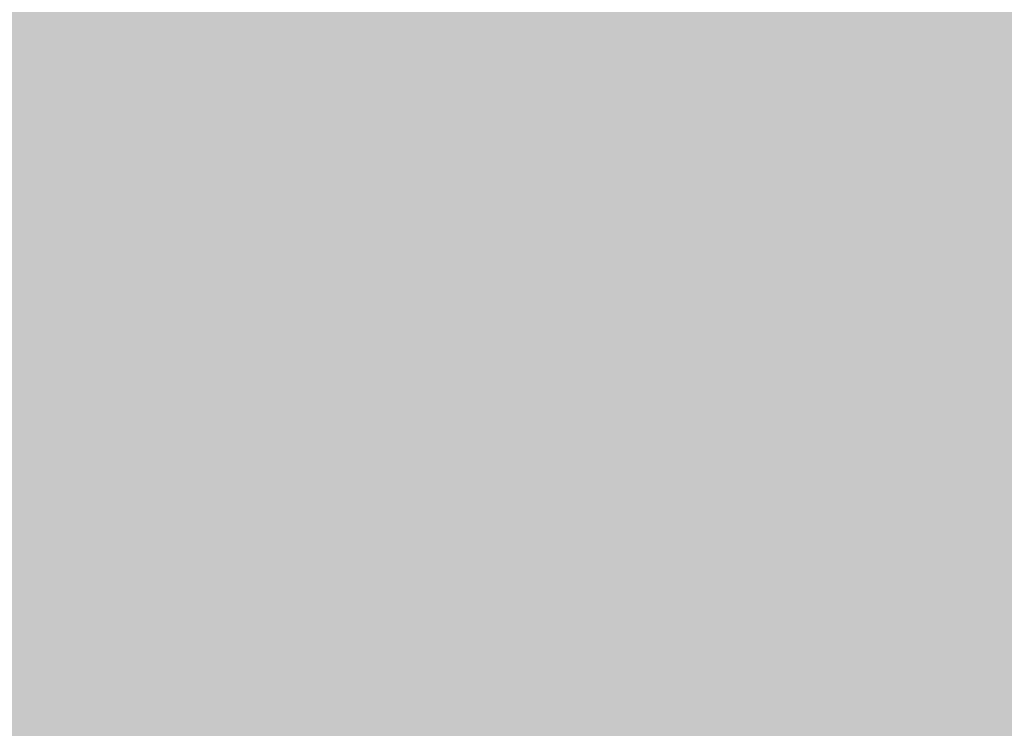
# Model space of a CAD drawing. Units: feet. Extents: x 3168 to 4724, y 827 to 1477.
# Tile 173 of 256: x 3303.032 to 3307.378, y 1093.654 to 1096.781. Entities that reach past the tile are written whole.
import ezdxf

# ---------------------------------------------------------------- set-up
doc = ezdxf.new("R2010")
doc.units = ezdxf.units.FT
doc.layers.add('A-ELEV-PATT', color=8, linetype='Continuous', lineweight=13)

msp = doc.modelspace()

# ---------------------------------------------------------------- hatches: boundary and pattern name
at = {"layer": 'A-ELEV-PATT'}
h = msp.add_hatch(color=256, dxfattribs=at)
h.dxf.hatch_style = 1
edge = h.paths.add_edge_path()
edge.add_ellipse((3552.9058, 979.2201), major_axis=(36.7449, 0), ratio=0.4848485, start_angle=0, end_angle=360)
edge = h.paths.add_edge_path()
edge.add_ellipse((3559.8916, 929.2523), major_axis=(36.7449, 0), ratio=0.4848485, start_angle=0, end_angle=360)
edge = h.paths.add_edge_path()
edge.add_line((3299.3168, 1198.6061), (3479.9167, 1198.6061))
edge.add_line((3479.9167, 1198.6061), (3479.9167, 1209.8686))
edge.add_spline(control_points=[(3479.9167, 1209.8686), (3464.3012, 1209.8686), (3448.6856, 1209.8686), (3410.9491, 1209.8686), (3388.8282, 1209.8686), (3355.6469, 1209.8686), (3344.5864, 1209.8686), (3327.9957, 1209.8686), (3322.4655, 1209.8686), (3314.1702, 1209.8686), (3311.4051, 1209.8686), (3307.2574, 1209.8686), (3305.8748, 1209.8686), (3303.801, 1209.8686), (3303.1097, 1209.8686), (3302.0728, 1209.8686), (3301.7272, 1209.8686), (3301.2087, 1209.8686), (3301.0359, 1209.8686), (3300.7767, 1209.8686), (3300.6903, 1209.8686), (3300.5606, 1209.8686), (3300.5174, 1209.8686), (3300.4526, 1209.8686), (3300.431, 1209.8686), (3300.3986, 1209.8686), (3300.3878, 1209.8686), (3300.3662, 1209.8686), (3300.3457, 1209.8686), (3300.3455, 1209.8686), (3300.3455, 1209.8686), (3300.3433, 1209.8686), (3300.3411, 1209.8686), (3300.3379, 1209.8686), (3300.3368, 1209.8686), (3300.3339, 1209.8686), (3300.3321, 1209.8686), (3300.3255, 1209.8686), (3300.3207, 1209.8686), (3300.3109, 1209.8686), (3300.306, 1209.8686), (3300.2905, 1209.8686), (3300.28, 1209.8686), (3300.2324, 1209.8688), (3300.1953, 1209.869), (3299.9511, 1209.8706), (3299.7448, 1209.8743), (3299.4368, 1209.8833), (3299.3344, 1209.8868), (3299.1811, 1209.8929), (3299.13, 1209.8951), (3298.6522, 1209.9168), (3298.2295, 1209.9457), (3297.6016, 1210.0024), (3297.3934, 1210.0235), (3297.0827, 1210.0583), (3296.9793, 1210.0705), (3296.293, 1210.1549), (3295.7181, 1210.2434), (3294.8687, 1210.3989), (3294.5877, 1210.4545), (3294.1693, 1210.5433), (3294.0304, 1210.5739), (3291.7071, 1211.1012), (3289.6536, 1211.8134), (3285.7763, 1213.564), (3283.9514, 1214.6035), (3280.5122, 1216.9801), (3278.8972, 1218.3176), (3276.3799, 1220.8295), (3275.416, 1221.9177), (3274.0393, 1223.7077), (3273.581, 1224.3495), (3273.1432, 1225.0163)], knot_values=[39.119033, 39.119033, 39.119033, 39.119033, 39.286353, 39.286353, 39.523379, 39.523379, 39.641892, 39.641892, 39.701148, 39.701148, 39.730777, 39.730777, 39.745591, 39.745591, 39.752998, 39.752998, 39.756701, 39.756701, 39.758553, 39.758553, 39.759479, 39.759479, 39.759942, 39.759942, 39.760173, 39.760173, 39.760289, 39.760289, 39.760405, 39.760405, 39.760463, 39.760463, 39.763389, 39.763389, 39.764851, 39.764851, 39.767304, 39.767304, 39.773825, 39.773825, 39.78057, 39.78057, 39.79477, 39.79477, 39.845194, 39.845194, 40.126715, 40.126715, 40.267476, 40.267476, 40.337856, 40.337856, 40.927023, 40.927023, 41.221606, 41.221606, 41.368898, 41.368898, 42.202622, 42.202622, 42.619485, 42.619485, 42.827916, 42.827916, 46.118323, 46.118323, 49.408731, 49.408731, 52.699139, 52.699139, 54.927489, 54.927489, 56.104228, 56.104228, 56.104228, 56.104228], weights=[1, 1, 1, 1, 1, 1, 1, 1, 1, 1, 1, 1, 1, 1, 1, 1, 1, 1, 1, 1, 1, 1, 1, 1, 1, 1, 1, 1, 1, 1, 1, 1, 1, 1, 1, 1, 1, 1, 1, 1, 1, 1, 1, 1, 1, 1, 1, 1, 1, 1, 1, 1, 1, 1, 1, 1, 1, 1, 1, 1, 1, 1, 1, 1, 1, 1, 1, 1, 1, 1, 1, 1, 1, 1], degree=3, periodic=0)
edge.add_line((3273.1432, 1225.0163), (3273.1432, 1099.0163))
edge.add_line((3273.1432, 1099.0163), (3299.3168, 1099.0163))
edge.add_line((3299.3168, 1099.0163), (3299.3168, 1198.6061))
edge = h.paths.add_edge_path()
edge.add_line((3304.7584, 1324.1581), (3479.9167, 1324.1581))
edge.add_line((3479.9167, 1324.1581), (3479.9167, 1335.7146))
edge.add_line((3479.9167, 1335.7146), (3269.1616, 1335.7146))
edge.add_spline(control_points=[(3269.1616, 1335.7146), (3264.0242, 1335.7146), (3258.3641, 1328.9582), (3259.2643, 1323.9003)], knot_values=[0, 0, 0, 0, 15.412191, 15.412191, 15.412191, 15.412191], degree=3, periodic=0)
edge.add_line((3259.2643, 1323.9003), (3265.5168, 1288.7691))
edge.add_line((3265.5168, 1288.7691), (3275.2651, 1261.5456))
edge.add_line((3275.2651, 1261.5456), (3304.7584, 1261.5456))
edge.add_line((3304.7584, 1261.5456), (3304.7584, 1324.1581))
h = msp.add_hatch(color=256, dxfattribs=at)
h.dxf.hatch_style = 1
h.paths.add_polyline_path([(3384.5252, 1099.0163), (3335.0292, 1099.0163), (3299.3168, 1099.0163), (3273.1432, 1099.0163), (3217.5654, 1099.0163), (3168.0693, 827.1163), (3335.0292, 827.1163)])

doc.saveas('drawing.dxf')
